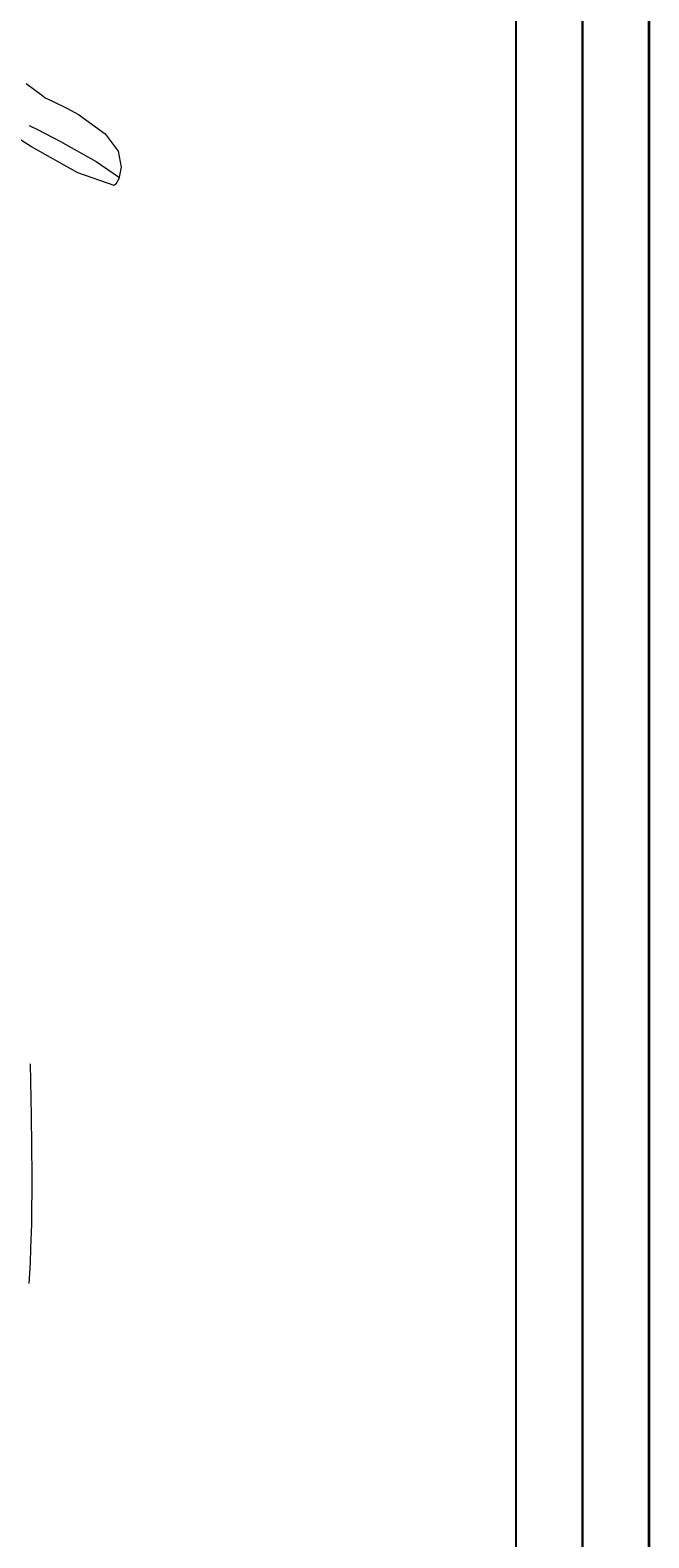
# Model space of a CAD drawing. Units: inches. Extents: x -16 to 587, y -783 to 64.
# Tile 5 of 14: x 195 to 237, y -697 to -595. Entities that reach past the tile are written whole.
import ezdxf

# ---------------------------------------------------------------- set-up
doc = ezdxf.new("R2010")
doc.units = ezdxf.units.IN
doc.header["$MEASUREMENT"] = 0
for name, color, linetype, lineweight in [('A-ANNO-DIMS', 2, 'Continuous', 18), ('A-SITE-VEHC', 8, 'Continuous', 13), ('A-SITE-WALL', 7, 'Continuous', 30), ('A-WALL', 7, 'Continuous', 35)]:
    doc.layers.add(name, color=color, linetype=linetype, lineweight=lineweight)
doc.styles.get("Standard").update_dxf_attribs({"font": 'arial.ttf'})
doc.dimstyles.get("Standard").update_dxf_attribs({"dimtxt": 0.18, "dimasz": 0.18, "dimexe": 0.18, "dimexo": 0.0625, "dimgap": 0.09, "dimtad": 0, "dimtih": 1, "dimtoh": 1, "dimdec": 0, "dimzin": 0, "dimdsep": 46, "dimlunit": 3, "dimtxsty": 'Standard', "dimcen": 0.09, "dimadec": 0, "dimazin": 0, "dimtfac": 1, "dimtdec": 0, "dimtofl": 0, "dimtmove": 0, "dimatfit": 3, "dimfxl": 1, "dimtolj": 1, "dimtzin": 0, "dimarcsym": 0})

# ---------------------------------------------------------------- blocks, each defined once
blk = doc.blocks.new('*D56')
at = {"layer": 'A-ANNO-DIMS', "color": 0, "lineweight": -2, "transparency": 16777216}
for p, q in [((118.08, -728.49), (118.08, 63.78)), ((118.26, 63.6), (172.75, 63.6)), ((227.9, 63.6), (173.41, 63.6)), ((228.08, -728.49), (228.08, 63.78))]:
    blk.add_line(p, q, dxfattribs=at)
at = {"layer": 'A-ANNO-DIMS', "color": 0, "transparency": 16777216}
for points in [[(118.26, 63.63), (118.26, 63.57), (118.08, 63.6)], [(227.9, 63.63), (227.9, 63.57), (228.08, 63.6)]]:
    blk.add_solid(points, dxfattribs=at)
at = {"layer": 'Defpoints', "color": 0, "transparency": 16777216}
for p in [(228.08, 63.6), (118.08, -728.55), (228.08, -728.55)]:
    blk.add_point(p, dxfattribs=at)
at = {"layer": 'A-ANNO-DIMS', "color": 0, "transparency": 16777216, "insert": (173.08, 63.6), "char_height": 0.18, "attachment_point": 5}
blk.add_mtext('\\A1;9\'-2"', dxfattribs=at)

msp = doc.modelspace()

# ---------------------------------------------------------------- linework, layer by layer
at = {"layer": 'A-SITE-VEHC'}
for p, q in [((194.83, -598.72), (195.87, -599.5)), ((195.87, -599.5), (196.12, -599.69)), ((196.12, -599.69), (196.62, -599.93)), ((196.62, -599.93), (197.62, -600.43)), ((197.62, -600.43), (198.37, -600.82)), ((198.37, -600.82), (200.18, -602.15)), ((195.19, -603.03), (193.64, -602.06)), ((195.02, -601.58), (195.65, -601.88)), ((195.65, -601.88), (197.15, -602.66)), ((200.18, -602.15), (201.07, -603.32)), ((198.33, -604.79), (195.19, -603.03)), ((197.15, -602.66), (199.57, -604.01)), ((201.07, -603.32), (201.27, -604.4)), ((199.57, -604.01), (201.15, -605.11)), ((201.27, -604.4), (201.12, -605.2)), ((200.79, -605.64), (198.33, -604.79)), ((201.12, -605.2), (200.9, -605.56)), ((200.9, -605.56), (200.79, -605.64)), ((195.09, -665.23), (195.17, -668.76)), ((195.17, -668.76), (195.22, -672.84)), ((195.22, -672.84), (195.18, -676.1)), ((195.18, -676.1), (195.13, -677.73)), ((195.13, -677.73), (195.1, -678.73)), ((195.1, -678.73), (195.01, -680.13))]:
    msp.add_line(p, q, dxfattribs=at)
at = {"layer": 'A-SITE-WALL'}
msp.add_line((232.58, -543.55), (232.58, -728.55), dxfattribs=at)
at = {"layer": 'A-WALL'}
msp.add_line((237.08, 19.45), (237.08, -737.55), dxfattribs=at)

# ---------------------------------------------------------------- dimensions: what is measured, and where the dimension line sits
at = {"layer": 'A-ANNO-DIMS'}
dim = msp.add_linear_dim(base=(228.08, 63.6), p1=(118.08, -728.55), p2=(228.08, -728.55), dimstyle='Standard', override={"dimdec": 1, "dimlfac": 1, "dimrnd": 0, "dimzin": 1, "dimdsep": 46, "dimlunit": 4, "dimfrac": 2}, dxfattribs=at)
dim.commit()
dim.dimension.update_dxf_attribs({"geometry": '*D56', "text_midpoint": (173.08, 63.6)})

doc.saveas('drawing.dxf')
